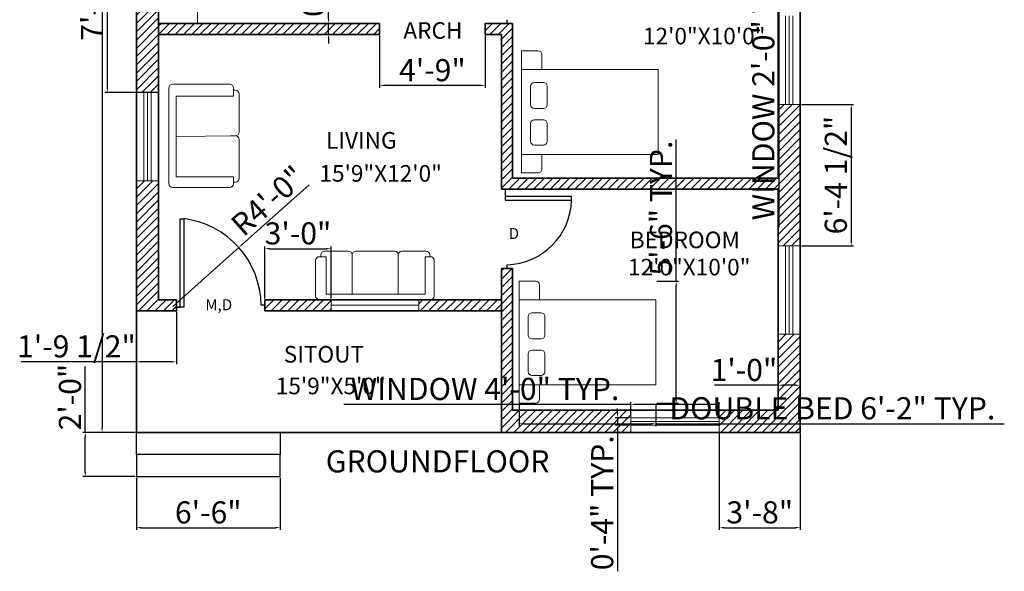
# Model space of a CAD drawing. Units: inches. Extents: x 2105 to 2639, y 1718 to 2373.
# Tile 1 of 2: x 2105 to 2639, y 1718 to 2017. Entities that reach past the tile are written whole.
import ezdxf

# ---------------------------------------------------------------- set-up
doc = ezdxf.new("R2010")
doc.units = ezdxf.units.IN
for name, color, linetype, lineweight in [('A-ANNO-DIMS', 2, 'Continuous', 18), ('A-ANNO-TEXT', 7, 'Continuous', 18), ('A-AREA-IDEN', 7, 'Continuous', 18), ('A-DOOR', 3, 'Continuous', 25), ('A-FLOR-CASE', 9, 'Continuous', 18), ('A-FLOR-STRS', 7, 'Continuous', 25), ('A-FURN', 8, 'Continuous', 18), ('A-GLAZ', 4, 'Continuous', 18), ('A-WALL', 120, 'Continuous', 35), ('A-WALL-PATT', 120, 'Continuous', 13)]:
    doc.layers.add(name, color=color, linetype=linetype, lineweight=lineweight)
doc.styles.get("Standard").update_dxf_attribs({"font": 'arial.ttf'})
doc.dimstyles.new('ISO-25', dxfattribs={"dimtxt": 12, "dimasz": 2.5, "dimexe": 1.25, "dimexo": 0.625, "dimtad": 1, "dimdec": 0, "dimlunit": 3, "dimtxsty": 'Standard', "dimcen": 2.5, "dimadec": 0, "dimazin": 0, "dimtfac": 1, "dimtdec": 0, "dimtmove": 0, "dimatfit": 3, "dimfxl": 1, "dimarcsym": 0})

# ---------------------------------------------------------------- blocks, each defined once
blk = doc.blocks.new('*D2')
at = {"layer": 'A-ANNO-DIMS', "color": 0, "lineweight": -2, "transparency": 16777216}
for p, q in [((2167.25, 2273.29), (2148.02, 2273.29)), ((2149.27, 2270.79), (2149.27, 1795.79)), ((2167.25, 1793.29), (2148.02, 1793.29))]:
    blk.add_line(p, q, dxfattribs=at)
at = {"layer": 'A-ANNO-DIMS', "color": 0, "transparency": 16777216}
for points in [[(2148.85, 2270.79), (2149.68, 2270.79), (2149.27, 2273.29)], [(2148.85, 1795.79), (2149.68, 1795.79), (2149.27, 1793.29)]]:
    blk.add_solid(points, dxfattribs=at)
at = {"layer": 'Defpoints', "color": 0, "transparency": 16777216}
for p in [(2167.87, 2273.29), (2149.27, 1793.29), (2167.87, 1793.29)]:
    blk.add_point(p, dxfattribs=at)
at = {"layer": 'A-ANNO-DIMS', "color": 0, "transparency": 16777216, "insert": (2142.52, 2033.29), "char_height": 12, "attachment_point": 5, "rotation": 90}
blk.add_mtext("40'", dxfattribs=at)
blk = doc.blocks.new('WIN-GLAZ-48IN')
for p, q in [((0, 4), (48, 4)), ((0, 2), (48, 2)), ((0, 0), (48, 0))]:
    blk.add_line(p, q)
blk = doc.blocks.new('DOOR-LEAF-36IN')
for p, q in [((2, 36), (0, 36)), ((0, 36), (0, 0)), ((2, 0), (2, 36)), ((0, 0), (2, 0))]:
    blk.add_line(p, q)
blk = doc.blocks.new('BED-DOUBLE')
for points in [[(0, 56.21), (11, 56.21), (11, 64.21, 0.414214), (9, 66.21), (0, 66.21)], [(6.91, 49.06), (11.92, 49.06, -0.414214), (13.92, 47.06), (13.92, 36.95, -0.414214), (11.92, 34.95), (6.91, 34.95, -0.414214), (4.91, 36.95), (4.91, 47.06, -0.414214)], [(6.91, 28.81), (11.92, 28.81, -0.414214), (13.92, 26.81), (13.92, 17.11, -0.414214), (11.92, 15.11), (6.91, 15.11, -0.414214), (4.91, 17.11), (4.91, 26.81, -0.414214)], [(0, 10), (11, 10), (11, 2, -0.414214), (9, 0), (0, 0)]]:
    blk.add_lwpolyline(points, format="xyb", close=True)
blk.add_lwpolyline([(0, 56.21), (74.08, 56.21), (74.08, 10), (0, 10)], close=True)
blk = doc.blocks.new('*D8')
at = {"layer": 'A-ANNO-DIMS', "color": 0, "lineweight": -2, "transparency": 16777216}
for p, q in [((2435.99, 1808.49), (2280.39, 1808.49)), ((2435.99, 1801.92), (2435.99, 1809.74)), ((2481.49, 1808.49), (2438.49, 1808.49)), ((2483.99, 1801.92), (2483.99, 1809.74))]:
    blk.add_line(p, q, dxfattribs=at)
at = {"layer": 'A-ANNO-DIMS', "color": 0, "transparency": 16777216}
for points in [[(2438.49, 1808.91), (2438.49, 1808.08), (2435.99, 1808.49)], [(2481.49, 1808.91), (2481.49, 1808.08), (2483.99, 1808.49)]]:
    blk.add_solid(points, dxfattribs=at)
at = {"layer": 'Defpoints', "color": 0, "transparency": 16777216}
for p in [(2435.99, 1808.49), (2435.99, 1801.29), (2483.99, 1801.29)]:
    blk.add_point(p, dxfattribs=at)
at = {"layer": 'A-ANNO-DIMS', "color": 0, "transparency": 16777216, "insert": (2356.94, 1815.33), "char_height": 12, "attachment_point": 5}
blk.add_mtext('WINDOW 4\'-0" TYP.', dxfattribs=at)
blk = doc.blocks.new('*D9')
at = {"layer": 'A-ANNO-DIMS', "color": 0, "lineweight": -2, "transparency": 16777216}
for p, q in [((2428.79, 1803.79), (2428.79, 1806.29)), ((2435.37, 1801.29), (2427.54, 1801.29)), ((2428.79, 1801.29), (2428.79, 1797.29)), ((2435.37, 1797.29), (2427.54, 1797.29)), ((2428.79, 1794.79), (2428.79, 1717.9))]:
    blk.add_line(p, q, dxfattribs=at)
at = {"layer": 'A-ANNO-DIMS', "color": 0, "transparency": 16777216}
for points in [[(2428.37, 1803.79), (2429.21, 1803.79), (2428.79, 1801.29)], [(2428.37, 1794.79), (2429.21, 1794.79), (2428.79, 1797.29)]]:
    blk.add_solid(points, dxfattribs=at)
at = {"layer": 'Defpoints', "color": 0, "transparency": 16777216}
for p in [(2435.99, 1801.29), (2428.79, 1797.29), (2435.99, 1797.29)]:
    blk.add_point(p, dxfattribs=at)
at = {"layer": 'A-ANNO-DIMS', "color": 0, "transparency": 16777216, "insert": (2422.04, 1755.09), "char_height": 12, "attachment_point": 5, "rotation": 90}
blk.add_mtext('0\'-4" TYP.', dxfattribs=at)
blk = doc.blocks.new('*D10')
at = {"layer": 'A-ANNO-DIMS', "color": 0, "lineweight": -2, "transparency": 16777216}
for p, q in [((2519.25, 2084.29), (2515.02, 2084.29)), ((2516.27, 2081.79), (2516.27, 2062.79)), ((2519.25, 2060.29), (2515.02, 2060.29)), ((2516.27, 2060.29), (2516.27, 1904.69))]:
    blk.add_line(p, q, dxfattribs=at)
at = {"layer": 'A-ANNO-DIMS', "color": 0, "transparency": 16777216}
for points in [[(2515.86, 2081.79), (2516.69, 2081.79), (2516.27, 2084.29)], [(2515.86, 2062.79), (2516.69, 2062.79), (2516.27, 2060.29)]]:
    blk.add_solid(points, dxfattribs=at)
at = {"layer": 'Defpoints', "color": 0, "transparency": 16777216}
for p in [(2519.87, 2084.29), (2516.27, 2060.29), (2519.87, 2060.29)]:
    blk.add_point(p, dxfattribs=at)
at = {"layer": 'A-ANNO-DIMS', "color": 0, "transparency": 16777216, "insert": (2509.44, 1981.24), "char_height": 12, "attachment_point": 5, "rotation": 90}
blk.add_mtext('WINDOW 2\'-0" TYP.', dxfattribs=at)
blk = doc.blocks.new('*D16')
at = {"layer": 'A-ANNO-DIMS', "color": 0, "lineweight": -2, "transparency": 16777216}
for p, q in [((2375.44, 1808.49), (2375.44, 1796.76)), ((2449.53, 1808.49), (2449.53, 1796.76)), ((2377.94, 1798.01), (2447.03, 1798.01)), ((2449.53, 1798.01), (2638.55, 1798.01))]:
    blk.add_line(p, q, dxfattribs=at)
at = {"layer": 'A-ANNO-DIMS', "color": 0, "transparency": 16777216}
for points in [[(2377.94, 1798.42), (2377.94, 1797.59), (2375.44, 1798.01)], [(2447.03, 1798.42), (2447.03, 1797.59), (2449.53, 1798.01)]]:
    blk.add_solid(points, dxfattribs=at)
at = {"layer": 'Defpoints', "color": 0, "transparency": 16777216}
for p in [(2375.44, 1809.12), (2449.53, 1809.12), (2449.53, 1798.01)]:
    blk.add_point(p, dxfattribs=at)
at = {"layer": 'A-ANNO-DIMS', "color": 0, "transparency": 16777216, "insert": (2545.29, 1804.84), "char_height": 12, "attachment_point": 5}
blk.add_mtext('DOUBLE BED 6\'-2" TYP.', dxfattribs=at)
blk = doc.blocks.new('*D17')
at = {"layer": 'A-ANNO-DIMS', "color": 0, "lineweight": -2, "transparency": 16777216}
for p, q in [((2460.64, 1875.33), (2460.64, 1952.23)), ((2450.15, 1875.33), (2461.89, 1875.33)), ((2460.64, 1811.62), (2460.64, 1872.83)), ((2450.15, 1809.12), (2461.89, 1809.12))]:
    blk.add_line(p, q, dxfattribs=at)
at = {"layer": 'A-ANNO-DIMS', "color": 0, "transparency": 16777216}
for points in [[(2460.22, 1872.83), (2461.06, 1872.83), (2460.64, 1875.33)], [(2460.22, 1811.62), (2461.06, 1811.62), (2460.64, 1809.12)]]:
    blk.add_solid(points, dxfattribs=at)
at = {"layer": 'Defpoints', "color": 0, "transparency": 16777216}
for p in [(2449.53, 1875.33), (2460.64, 1875.33), (2449.53, 1809.12)]:
    blk.add_point(p, dxfattribs=at)
at = {"layer": 'A-ANNO-DIMS', "color": 0, "transparency": 16777216, "insert": (2453.89, 1915.03), "char_height": 12, "attachment_point": 5, "rotation": 90}
blk.add_mtext('5\'-6" TYP.', dxfattribs=at)
blk = doc.blocks.new('*D18')
at = {"layer": 'A-ANNO-DIMS', "color": 0, "lineweight": -2, "transparency": 16777216}
for p, q in [((2167.87, 1768.67), (2167.87, 1740.34)), ((2245.87, 1768.67), (2245.87, 1740.34)), ((2170.37, 1741.59), (2243.37, 1741.59))]:
    blk.add_line(p, q, dxfattribs=at)
at = {"layer": 'A-ANNO-DIMS', "color": 0, "transparency": 16777216}
for points in [[(2170.37, 1742.01), (2170.37, 1741.18), (2167.87, 1741.59)], [(2243.37, 1742.01), (2243.37, 1741.18), (2245.87, 1741.59)]]:
    blk.add_solid(points, dxfattribs=at)
at = {"layer": 'Defpoints', "color": 0, "transparency": 16777216}
for p in [(2167.87, 1769.29), (2245.87, 1769.29), (2245.87, 1741.59)]:
    blk.add_point(p, dxfattribs=at)
at = {"layer": 'A-ANNO-DIMS', "color": 0, "transparency": 16777216, "insert": (2206.87, 1748.34), "char_height": 12, "attachment_point": 5}
blk.add_mtext('6\'-6"', dxfattribs=at)
blk = doc.blocks.new('*D19')
at = {"layer": 'A-ANNO-DIMS', "color": 0, "lineweight": -2, "transparency": 16777216}
for p, q in [((2140.17, 1793.29), (2140.17, 1829.15)), ((2167.25, 1793.29), (2138.92, 1793.29)), ((2140.17, 1771.79), (2140.17, 1790.79)), ((2167.25, 1769.29), (2138.92, 1769.29))]:
    blk.add_line(p, q, dxfattribs=at)
at = {"layer": 'A-ANNO-DIMS', "color": 0, "transparency": 16777216}
for points in [[(2139.76, 1790.79), (2140.59, 1790.79), (2140.17, 1793.29)], [(2139.76, 1771.79), (2140.59, 1771.79), (2140.17, 1769.29)]]:
    blk.add_solid(points, dxfattribs=at)
at = {"layer": 'Defpoints', "color": 0, "transparency": 16777216}
for p in [(2140.17, 1793.29), (2167.87, 1793.29), (2167.87, 1769.29)]:
    blk.add_point(p, dxfattribs=at)
at = {"layer": 'A-ANNO-DIMS', "color": 0, "transparency": 16777216, "insert": (2133.42, 1812.47), "char_height": 12, "attachment_point": 5, "rotation": 90}
blk.add_mtext('2\'-0"', dxfattribs=at)
blk = doc.blocks.new('*D26')
at = {"layer": 'A-ANNO-DIMS', "color": 0, "lineweight": -2, "transparency": 16777216}
for p, q in [((2528.5, 1971.31), (2556.82, 1971.31)), ((2555.57, 1968.81), (2555.57, 1897.09)), ((2528.5, 1894.59), (2556.82, 1894.59))]:
    blk.add_line(p, q, dxfattribs=at)
at = {"layer": 'A-ANNO-DIMS', "color": 0, "transparency": 16777216}
for points in [[(2555.16, 1968.81), (2555.99, 1968.81), (2555.57, 1971.31)], [(2555.16, 1897.09), (2555.99, 1897.09), (2555.57, 1894.59)]]:
    blk.add_solid(points, dxfattribs=at)
at = {"layer": 'Defpoints', "color": 0, "transparency": 16777216}
for p in [(2527.87, 1971.31), (2527.87, 1894.59), (2555.57, 1894.59)]:
    blk.add_point(p, dxfattribs=at)
at = {"layer": 'A-ANNO-DIMS', "color": 0, "transparency": 16777216, "insert": (2548.74, 1932.95), "char_height": 12, "attachment_point": 5, "rotation": 90}
blk.add_mtext('6\'-4 1/2"', dxfattribs=at)
blk = doc.blocks.new('*D27')
at = {"layer": 'A-ANNO-DIMS', "color": 0, "lineweight": -2, "transparency": 16777216}
for p, q in [((2483.99, 1792.67), (2483.99, 1740.34)), ((2527.87, 1792.67), (2527.87, 1740.34)), ((2486.49, 1741.59), (2525.37, 1741.59))]:
    blk.add_line(p, q, dxfattribs=at)
at = {"layer": 'A-ANNO-DIMS', "color": 0, "transparency": 16777216}
for points in [[(2486.49, 1742.01), (2486.49, 1741.18), (2483.99, 1741.59)], [(2525.37, 1742.01), (2525.37, 1741.18), (2527.87, 1741.59)]]:
    blk.add_solid(points, dxfattribs=at)
at = {"layer": 'Defpoints', "color": 0, "transparency": 16777216}
for p in [(2483.99, 1793.29), (2527.87, 1793.29), (2527.87, 1741.59)]:
    blk.add_point(p, dxfattribs=at)
at = {"layer": 'A-ANNO-DIMS', "color": 0, "transparency": 16777216, "insert": (2505.93, 1748.35), "char_height": 12, "attachment_point": 5}
blk.add_mtext('3\'-8"', dxfattribs=at)
blk = doc.blocks.new('*D31')
at = {"layer": 'A-ANNO-DIMS', "color": 0, "lineweight": -2, "transparency": 16777216}
for p, q in [((2179.25, 2070.06), (2150.92, 2070.06)), ((2152.17, 1980.35), (2152.17, 2067.56)), ((2179.25, 1977.85), (2150.92, 1977.85))]:
    blk.add_line(p, q, dxfattribs=at)
at = {"layer": 'A-ANNO-DIMS', "color": 0, "transparency": 16777216}
for points in [[(2151.76, 2067.56), (2152.59, 2067.56), (2152.17, 2070.06)], [(2151.76, 1980.35), (2152.59, 1980.35), (2152.17, 1977.85)]]:
    blk.add_solid(points, dxfattribs=at)
at = {"layer": 'Defpoints', "color": 0, "transparency": 16777216}
for p in [(2152.17, 2070.06), (2179.87, 2070.06), (2179.87, 1977.85)]:
    blk.add_point(p, dxfattribs=at)
at = {"layer": 'A-ANNO-DIMS', "color": 0, "transparency": 16777216, "insert": (2145.42, 2023.95), "char_height": 12, "attachment_point": 5, "rotation": 90}
blk.add_mtext('7\'-8"', dxfattribs=at)
blk = doc.blocks.new('*D32')
at = {"layer": 'A-ANNO-DIMS', "color": 0, "lineweight": -2, "transparency": 16777216}
for p, q in [((2167.87, 1858.67), (2167.87, 1830.34)), ((2189.6, 1858.67), (2189.6, 1830.34)), ((2167.87, 1831.59), (2105.39, 1831.59)), ((2187.1, 1831.59), (2170.37, 1831.59))]:
    blk.add_line(p, q, dxfattribs=at)
at = {"layer": 'A-ANNO-DIMS', "color": 0, "transparency": 16777216}
for points in [[(2170.37, 1832.01), (2170.37, 1831.18), (2167.87, 1831.59)], [(2187.1, 1832.01), (2187.1, 1831.18), (2189.6, 1831.59)]]:
    blk.add_solid(points, dxfattribs=at)
at = {"layer": 'Defpoints', "color": 0, "transparency": 16777216}
for p in [(2167.87, 1859.29), (2189.6, 1859.29), (2167.87, 1831.59)]:
    blk.add_point(p, dxfattribs=at)
at = {"layer": 'A-ANNO-DIMS', "color": 0, "transparency": 16777216, "insert": (2135.38, 1838.42), "char_height": 12, "attachment_point": 5}
blk.add_mtext('1\'-9 1/2"', dxfattribs=at)
blk = doc.blocks.new('*D33')
at = {"layer": 'A-ANNO-DIMS', "color": 0, "lineweight": -2, "transparency": 16777216}
for p, q in [((2237.6, 1865.92), (2237.6, 1894.24)), ((2240.1, 1892.99), (2270.94, 1892.99)), ((2273.44, 1865.92), (2273.44, 1894.24))]:
    blk.add_line(p, q, dxfattribs=at)
at = {"layer": 'A-ANNO-DIMS', "color": 0, "transparency": 16777216}
for points in [[(2240.1, 1893.41), (2240.1, 1892.58), (2237.6, 1892.99)], [(2270.94, 1893.41), (2270.94, 1892.58), (2273.44, 1892.99)]]:
    blk.add_solid(points, dxfattribs=at)
at = {"layer": 'Defpoints', "color": 0, "transparency": 16777216}
for p in [(2273.44, 1892.99), (2237.6, 1865.29), (2273.44, 1865.29)]:
    blk.add_point(p, dxfattribs=at)
at = {"layer": 'A-ANNO-DIMS', "color": 0, "transparency": 16777216, "insert": (2255.52, 1899.75), "char_height": 12, "attachment_point": 5}
blk.add_mtext('3\'-0"', dxfattribs=at)
blk = doc.blocks.new('*D34')
at = {"layer": 'A-ANNO-DIMS', "color": 0, "lineweight": -2, "transparency": 16777216}
for p, q in [((2299.8, 2008.67), (2299.8, 1980.34)), ((2357.02, 2008.67), (2357.02, 1980.34)), ((2354.52, 1981.59), (2302.3, 1981.59))]:
    blk.add_line(p, q, dxfattribs=at)
at = {"layer": 'A-ANNO-DIMS', "color": 0, "transparency": 16777216}
for points in [[(2302.3, 1982.01), (2302.3, 1981.18), (2299.8, 1981.59)], [(2354.52, 1982.01), (2354.52, 1981.18), (2357.02, 1981.59)]]:
    blk.add_solid(points, dxfattribs=at)
at = {"layer": 'Defpoints', "color": 0, "transparency": 16777216}
for p in [(2299.8, 2009.29), (2357.02, 2009.29), (2299.8, 1981.59)]:
    blk.add_point(p, dxfattribs=at)
at = {"layer": 'A-ANNO-DIMS', "color": 0, "transparency": 16777216, "insert": (2328.41, 1988.34), "char_height": 12, "attachment_point": 5}
blk.add_mtext('4\'-9"', dxfattribs=at)
blk = doc.blocks.new('*D37')
at = {"layer": 'A-ANNO-DIMS', "color": 0, "lineweight": -2, "transparency": 16777216}
for p, q in [((2515.87, 1845.96), (2515.87, 1817.64)), ((2527.87, 1845.96), (2527.87, 1817.64)), ((2515.87, 1818.89), (2481.35, 1818.89)), ((2525.37, 1818.89), (2518.37, 1818.89))]:
    blk.add_line(p, q, dxfattribs=at)
at = {"layer": 'A-ANNO-DIMS', "color": 0, "transparency": 16777216}
for points in [[(2518.37, 1819.3), (2518.37, 1818.47), (2515.87, 1818.89)], [(2525.37, 1819.3), (2525.37, 1818.47), (2527.87, 1818.89)]]:
    blk.add_solid(points, dxfattribs=at)
at = {"layer": 'Defpoints', "color": 0, "transparency": 16777216}
for p in [(2515.87, 1846.59), (2527.87, 1846.59), (2515.87, 1818.89)]:
    blk.add_point(p, dxfattribs=at)
at = {"layer": 'A-ANNO-DIMS', "color": 0, "transparency": 16777216, "insert": (2497.36, 1825.64), "char_height": 12, "attachment_point": 5}
blk.add_mtext('1\'-0"', dxfattribs=at)
blk = doc.blocks.new('*D38')
at = {"layer": 'A-ANNO-DIMS', "color": 0, "lineweight": -2, "transparency": 16777216}
for p, q in [((2272.1, 2017.79), (2272.1, 2053.44)), ((2299.18, 2015.29), (2270.85, 2015.29)), ((2272.1, 2009.29), (2272.1, 2015.29)), ((2299.18, 2009.29), (2270.85, 2009.29)), ((2272.1, 2006.79), (2272.1, 2004.29))]:
    blk.add_line(p, q, dxfattribs=at)
at = {"layer": 'A-ANNO-DIMS', "color": 0, "transparency": 16777216}
for points in [[(2271.69, 2017.79), (2272.52, 2017.79), (2272.1, 2015.29)], [(2271.69, 2006.79), (2272.52, 2006.79), (2272.1, 2009.29)]]:
    blk.add_solid(points, dxfattribs=at)
at = {"layer": 'Defpoints', "color": 0, "transparency": 16777216}
for p in [(2272.1, 2015.29), (2299.8, 2015.29), (2299.8, 2009.29)]:
    blk.add_point(p, dxfattribs=at)
at = {"layer": 'A-ANNO-DIMS', "color": 0, "transparency": 16777216, "insert": (2265.35, 2036.87), "char_height": 12, "attachment_point": 5, "rotation": 90}
blk.add_mtext('0\'-6"', dxfattribs=at)
blk = doc.blocks.new('*D41')
at = {"layer": 'A-ANNO-DIMS', "color": 0, "lineweight": -2, "transparency": 16777216}
for p, q in [((2261.51, 1927.71), (2225.26, 1895.32)), ((2187.61, 1861.67), (2223.4, 1893.65))]:
    blk.add_line(p, q, dxfattribs=at)
at = {"layer": 'A-ANNO-DIMS', "color": 0, "transparency": 16777216}
blk.add_solid([(2224.99, 1895.63), (2225.54, 1895.01), (2223.4, 1893.65)], dxfattribs=at)
at = {"layer": 'Defpoints', "color": 0, "transparency": 16777216}
for p in [(2223.4, 1893.65), (2187.61, 1861.67)]:
    blk.add_point(p, dxfattribs=at)
at = {"layer": 'A-ANNO-DIMS', "color": 0, "transparency": 16777216, "insert": (2240.37, 1917.88), "char_height": 12, "attachment_point": 5, "rotation": 41.7849}
blk.add_mtext('R4\'-0"', dxfattribs=at)

msp = doc.modelspace()

# ---------------------------------------------------------------- hatches: boundary and pattern name
at = {"layer": 'A-WALL-PATT'}
h = msp.add_hatch(dxfattribs=at)
h.set_pattern_fill('ANSI31', color=256)
h.paths.add_polyline_path([(2179.87, 2070.06), (2167.87, 2070.06), (2167.87, 1977.85), (2179.87, 1977.85)])
h = msp.add_hatch(dxfattribs=at)
h.set_pattern_fill('ANSI31', color=256)
h.paths.add_polyline_path([(2299.8, 2015.29), (2179.87, 2015.29), (2179.87, 2009.29), (2299.8, 2009.29)])
h = msp.add_hatch(dxfattribs=at)
h.set_pattern_fill('ANSI31', color=256)
h.paths.add_polyline_path([(2371.87, 2015.29), (2357.02, 2015.29), (2357.02, 2009.29), (2365.87, 2009.29), (2365.87, 1925.29), (2367.87, 1925.29), (2371.87, 1925.29), (2515.87, 1925.29), (2515.87, 1894.59), (2527.87, 1894.59), (2527.87, 1971.31), (2515.87, 1971.31), (2515.87, 1931.29), (2371.87, 1931.29)])
h = msp.add_hatch(dxfattribs=at)
h.set_pattern_fill('ANSI31', color=256)
h.paths.add_polyline_path([(2189.6, 1861.29), (2189.6, 1865.29), (2179.87, 1865.29), (2179.87, 1929.85), (2167.87, 1929.85), (2167.87, 1859.29), (2179.87, 1859.29), (2189.6, 1859.29)])
h = msp.add_hatch(dxfattribs=at)
h.set_pattern_fill('ANSI31', color=256)
h.paths.add_polyline_path([(2435.99, 1805.29), (2371.87, 1805.29), (2371.87, 1882.29), (2365.87, 1882.29), (2365.87, 1805.29), (2365.87, 1793.29), (2435.99, 1793.29)])
h = msp.add_hatch(dxfattribs=at)
h.set_pattern_fill('ANSI31', color=256)
h.paths.add_polyline_path([(2273.44, 1865.29), (2237.6, 1865.29), (2237.6, 1859.29), (2273.44, 1859.29)])
h = msp.add_hatch(dxfattribs=at)
h.set_pattern_fill('ANSI31', color=256)
h.paths.add_polyline_path([(2365.87, 1865.29), (2321.01, 1865.29), (2321.01, 1859.29), (2365.87, 1859.29)])
h = msp.add_hatch(dxfattribs=at)
h.set_pattern_fill('ANSI31', color=256)
h.paths.add_polyline_path([(2527.87, 1846.59), (2515.87, 1846.59), (2515.87, 1805.29), (2483.99, 1805.29), (2483.99, 1793.29), (2527.87, 1793.29)])

# ---------------------------------------------------------------- linework, layer by layer
at = {"layer": 'A-DOOR'}
for p, q in [((2368.87, 2015.29), (2368.87, 2017.29)), ((2371.87, 2015.29), (2368.87, 2015.29)), ((2365.87, 1925.29), (2367.87, 1925.29)), ((2367.87, 1925.29), (2367.87, 1921.29)), ((2191.6, 1861.29), (2191.6, 1909.29)), ((2191.6, 1909.29), (2193.6, 1909.29)), ((2193.6, 1909.29), (2193.6, 1861.29)), ((2368.87, 1882.29), (2368.87, 1884.29)), ((2189.6, 1859.29), (2189.6, 1861.29)), ((2189.6, 1861.29), (2191.6, 1861.29)), ((2193.6, 1861.29), (2190.6, 1861.29)), ((2237.6, 1862.29), (2235.6, 1862.29))]:
    msp.add_line(p, q, dxfattribs=at)
for centre, radius, start, end in [((2367.89, 1920.28), 36, 271.5702, 358.4298), ((2187.61, 1861.67), 48, 0.7449, 82.8241)]:
    msp.add_arc(centre, radius, start, end, dxfattribs=at)
at = {"layer": 'A-FLOR-CASE'}
msp.add_lwpolyline([(2179.87, 2015.29), (2201.1, 2015.29), (2201.1, 2060.06), (2179.87, 2060.06)], close=True, dxfattribs=at)
at = {"layer": 'A-FLOR-STRS'}
for p, q in [((2167.87, 1793.29), (2245.87, 1793.29)), ((2167.87, 1781.29), (2167.87, 1793.29)), ((2245.87, 1793.29), (2245.87, 1781.29)), ((2245.87, 1781.29), (2167.87, 1781.29)), ((2167.87, 1781.29), (2167.87, 1769.29)), ((2245.87, 1769.29), (2245.87, 1781.29)), ((2245.87, 1781.29), (2245.87, 1781.29)), ((2167.87, 1769.29), (2245.87, 1769.29))]:
    msp.add_line(p, q, dxfattribs=at)
at = {"layer": 'A-FURN'}
for p, q in [((2220.58, 1979.04), (2221.58, 1979.04)), ((2223.58, 1977.04), (2223.58, 1956.27)), ((2221.55, 1954.27), (2189.55, 1953.83)), ((2221.6, 1954.27), (2218.87, 1954.23)), ((2223.58, 1931.09), (2223.58, 1952.27)), ((2220.58, 1929.09), (2221.58, 1929.09)), ((2324.94, 1891.66), (2311.94, 1891.66)), ((2267.91, 1888.66), (2267.91, 1889.66)), ((2309.94, 1889.66), (2309.94, 1868.36)), ((2326.94, 1888.66), (2326.94, 1889.66))]:
    msp.add_line(p, q, dxfattribs=at)
for points in [[(2220.58, 1931.91), (2220.58, 1928.27, -0.414214), (2218.58, 1926.27), (2187.47, 1926.27, -0.414214), (2185.47, 1928.27), (2185.47, 1980.33, -0.414214), (2187.47, 1982.33), (2218.58, 1982.33, -0.414214), (2220.58, 1980.33), (2220.58, 1975.75)], [(2284.91, 1868.36), (2284.91, 1889.66, -0.414214), (2286.91, 1891.66), (2307.94, 1891.66, -0.414214), (2309.94, 1889.66), (2309.94, 1868.36), (2284.91, 1868.36), (2284.91, 1889.66, 0.414214), (2282.91, 1891.66), (2269.91, 1891.66)], [(2324.51, 1888.66), (2327.36, 1888.66, -0.414214), (2329.36, 1886.66), (2329.36, 1867.29, -0.414214), (2327.36, 1865.29), (2267.09, 1865.29, -0.414214), (2265.09, 1867.29), (2265.09, 1886.66, -0.414214), (2267.09, 1888.66), (2270.74, 1888.66)]]:
    msp.add_lwpolyline(points, format="xyb", dxfattribs=at)
for points in [[(2220.58, 1975.75), (2189.55, 1975.75), (2189.55, 1931.91), (2220.58, 1931.91)], [(2324.51, 1888.66), (2324.51, 1868.36), (2270.74, 1868.36), (2270.74, 1888.66)]]:
    msp.add_lwpolyline(points, dxfattribs=at)
for centre, start, end in [((2221.58, 1977.04), 0, 90), ((2221.58, 1952.27), 360, 90.7909), ((2221.58, 1956.27), 270.7909, 0), ((2221.58, 1931.09), 270, 360), ((2269.91, 1889.66), 90, 180), ((2311.94, 1889.66), 90, 180), ((2324.94, 1889.66), 0, 90)]:
    msp.add_arc(centre, 2, start, end, dxfattribs=at)
at = {"layer": 'A-GLAZ'}
for p, q in [((2167.87, 1977.85), (2179.87, 1977.85)), ((2527.87, 1971.31), (2515.87, 1971.31)), ((2167.87, 1929.85), (2179.87, 1929.85)), ((2527.87, 1894.59), (2515.87, 1894.59)), ((2273.44, 1865.29), (2273.44, 1859.29)), ((2321.01, 1865.29), (2321.01, 1859.29)), ((2273.44, 1862.29), (2321.01, 1862.29)), ((2527.87, 1846.59), (2515.87, 1846.59)), ((2435.99, 1793.29), (2435.99, 1805.29)), ((2483.99, 1793.29), (2483.99, 1805.29))]:
    msp.add_line(p, q, dxfattribs=at)
at = {"layer": 'A-WALL'}
for p, q in [((2179.87, 1865.29), (2179.87, 2129.29)), ((2515.87, 2054.29), (2515.87, 1931.29)), ((2179.87, 2015.29), (2299.8, 2015.29)), ((2299.8, 2015.29), (2299.8, 2009.29)), ((2357.02, 2015.29), (2371.87, 2015.29)), ((2357.02, 2015.29), (2357.02, 2009.29)), ((2371.87, 1931.29), (2371.87, 2015.29)), ((2179.87, 2009.29), (2299.8, 2009.29)), ((2357.02, 2009.29), (2365.87, 2009.29)), ((2365.87, 1925.29), (2365.87, 2009.29)), ((2515.87, 1931.29), (2371.87, 1931.29)), ((2371.87, 1925.29), (2365.87, 1925.29)), ((2515.87, 1925.29), (2371.87, 1925.29)), ((2515.87, 1925.29), (2515.87, 1805.29)), ((2365.87, 1805.29), (2365.87, 1882.29)), ((2371.87, 1882.29), (2365.87, 1882.29)), ((2371.87, 1805.29), (2371.87, 1882.29)), ((2179.87, 1865.29), (2189.6, 1865.29)), ((2189.6, 1865.29), (2189.6, 1859.29)), ((2237.6, 1865.29), (2237.6, 1859.29)), ((2237.6, 1865.29), (2365.87, 1865.29)), ((2179.87, 1859.29), (2167.87, 1859.29)), ((2179.87, 1859.29), (2189.6, 1859.29)), ((2237.6, 1859.29), (2365.87, 1859.29)), ((2365.87, 1805.29), (2365.87, 1793.29)), ((2515.87, 1805.29), (2371.87, 1805.29))]:
    msp.add_line(p, q, dxfattribs=at)
msp.add_lwpolyline([(2167.87, 2172.29), (2167.87, 2273.29), (2527.87, 2273.29), (2527.87, 1793.29), (2167.87, 1793.29), (2167.87, 2129.29)], dxfattribs=at)

# ---------------------------------------------------------------- block references
at = {"layer": 'A-DOOR', "rotation": 89.99999999999785}
msp.add_blockref('DOOR-LEAF-36IN', (2403.87, 1919.29), dxfattribs=at)
at = {"layer": 'A-FURN', "rotation": 0.0004994955271128}
msp.add_blockref('BED-DOUBLE', (2376.79, 1934.13), dxfattribs=at)
at = {"layer": 'A-FURN'}
msp.add_blockref('BED-DOUBLE', (2375.44, 1809.12), dxfattribs=at)
at = {"layer": 'A-GLAZ'}
for p, rotation in [((2519.87, 2019.31), 270.0000000000023), ((2175.87, 1929.85), 90.00000000000097), ((2519.87, 1894.59), 270.0000000000021), ((2483.99, 1801.29), 180)]:
    msp.add_blockref('WIN-GLAZ-48IN', p, dxfattribs=dict(at, rotation=rotation))

# ---------------------------------------------------------------- texts
at = {"layer": 'A-ANNO-TEXT'}
for tag, p, height in [('ARCH', (2312.67, 2006.92), 9), ('D', (2369.77, 1898.27), 6), ('M,D', (2205.29, 1859.59), 6), ('GROUNDFLOOR', (2270.57, 1771.58), 12)]:
    msp.add_attdef(tag, p, '', height=height, dxfattribs=at)
at = {"layer": 'A-AREA-IDEN'}
for tag, p in [('12\'0"X10\'0"', (2442.61, 2003.9)), ('LIVING', (2270.74, 1947.3)), ('15\'9"X12\'0"', (2267.16, 1929.38)), ('BEDROOM', (2435.44, 1893.27)), ('12\'0"X10\'0"', (2434.49, 1878.5)), ('SITOUT', (2247.79, 1831.2)), ('15\'9"X5\'0"', (2243.49, 1814))]:
    msp.add_attdef(tag, p, '', height=9, dxfattribs=at)

# ---------------------------------------------------------------- dimensions: what is measured, and where the dimension line sits
at = {"layer": 'A-ANNO-DIMS'}
for base, p1, p2, angle, override, picture, middle in [((2149.27, 1793.29), (2167.87, 2273.29), (2167.87, 1793.29), 90, {"dimclrd": 0, "dimclre": 0, "dimclrt": 0}, '*D2', (2142.52, 2033.29)), ((2152.17, 2070.06), (2179.87, 1977.85), (2179.87, 2070.06), 90, {"dimdec": 1, "dimlfac": 1, "dimrnd": 0, "dimzin": 1, "dimdsep": 46, "dimlunit": 4, "dimfrac": 2}, '*D31', (2145.42, 2023.95)), ((2272.1, 2015.29), (2299.8, 2009.29), (2299.8, 2015.29), 90, {"dimdec": 1, "dimlfac": 1, "dimrnd": 0, "dimzin": 1, "dimdsep": 46, "dimlunit": 4, "dimfrac": 2}, '*D38', (2265.35, 2036.87)), ((2299.8, 1981.59), (2357.02, 2009.29), (2299.8, 2009.29), 180, {"dimdec": 1, "dimlfac": 1, "dimrnd": 0, "dimzin": 1, "dimdsep": 46, "dimlunit": 4, "dimfrac": 2}, '*D34', (2328.41, 1988.34)), ((2555.57, 1894.59), (2527.87, 1971.31), (2527.87, 1894.59), 90, {"dimdec": 1, "dimlfac": 1, "dimrnd": 0, "dimzin": 1, "dimdsep": 46, "dimlunit": 4, "dimfrac": 2}, '*D26', (2548.74, 1932.95)), ((2167.87, 1831.59), (2189.6, 1859.29), (2167.87, 1859.29), 180, {"dimdec": 1, "dimlfac": 1, "dimrnd": 0, "dimzin": 1, "dimdsep": 46, "dimlunit": 4, "dimfrac": 2}, '*D32', (2135.38, 1838.42)), ((2515.87, 1818.89), (2527.87, 1846.59), (2515.87, 1846.59), 180, {"dimdec": 1, "dimlfac": 1, "dimrnd": 0, "dimzin": 1, "dimdsep": 46, "dimlunit": 4, "dimfrac": 2}, '*D37', (2497.36, 1825.64)), ((2140.17, 1793.29), (2167.87, 1769.29), (2167.87, 1793.29), 90, {"dimdec": 1, "dimlfac": 1, "dimrnd": 0, "dimzin": 1, "dimdsep": 46, "dimlunit": 4, "dimfrac": 2}, '*D19', (2133.42, 1812.47))]:
    dim = msp.add_linear_dim(base=base, p1=p1, p2=p2, angle=angle, dimstyle='ISO-25', override=override, dxfattribs=at)
    dim.commit()
    dim.dimension.update_dxf_attribs({"geometry": picture, "text_midpoint": middle})
for base, p1, p2, angle, text, picture, middle in [((2516.27, 2060.29), (2519.87, 2084.29), (2519.87, 2060.29), 270, 'WINDOW <> TYP.', '*D10', (2509.44, 1981.24)), ((2460.64, 1875.33), (2449.53, 1809.12), (2449.53, 1875.33), 90, '<> TYP.', '*D17', (2453.89, 1915.03)), ((2435.99, 1808.49), (2483.99, 1801.29), (2435.99, 1801.29), 180, 'WINDOW <> TYP.', '*D8', (2356.94, 1815.33)), ((2428.79, 1797.29), (2435.99, 1801.29), (2435.99, 1797.29), 270, '<> TYP.', '*D9', (2422.04, 1755.09))]:
    dim = msp.add_linear_dim(base=base, p1=p1, p2=p2, angle=angle, text=text, dimstyle='ISO-25', override={"dimdec": 1, "dimlfac": 1, "dimrnd": 0, "dimzin": 1, "dimdsep": 46, "dimlunit": 4, "dimfrac": 2}, dxfattribs=at)
    dim.commit()
    dim.dimension.update_dxf_attribs({"geometry": picture, "text_midpoint": middle})
dim = msp.add_radius_dim(center=(2187.61, 1861.67), mpoint=(2223.4, 1893.65), dimstyle='ISO-25', override={"dimdec": 1, "dimlfac": 1, "dimrnd": 0, "dimzin": 1, "dimdsep": 46, "dimlunit": 4, "dimfrac": 2}, dxfattribs=at)
dim.commit()
dim.dimension.update_dxf_attribs({"geometry": '*D41', "text_midpoint": (2244.87, 1912.84), "dimtype": 164})
for base, p1, p2, picture, middle in [((2273.44, 1892.99), (2237.6, 1865.29), (2273.44, 1865.29), '*D33', (2255.52, 1899.75)), ((2527.87, 1741.59), (2483.99, 1793.29), (2527.87, 1793.29), '*D27', (2505.93, 1748.35)), ((2245.87, 1741.59), (2167.87, 1769.29), (2245.87, 1769.29), '*D18', (2206.87, 1748.34))]:
    dim = msp.add_linear_dim(base=base, p1=p1, p2=p2, dimstyle='ISO-25', override={"dimdec": 1, "dimlfac": 1, "dimrnd": 0, "dimzin": 1, "dimdsep": 46, "dimlunit": 4, "dimfrac": 2}, dxfattribs=at)
    dim.commit()
    dim.dimension.update_dxf_attribs({"geometry": picture, "text_midpoint": middle})
dim = msp.add_linear_dim(base=(2449.53, 1798.01), p1=(2375.44, 1809.12), p2=(2449.53, 1809.12), text='DOUBLE BED <> TYP.', dimstyle='ISO-25', override={"dimdec": 1, "dimlfac": 1, "dimrnd": 0, "dimzin": 1, "dimdsep": 46, "dimlunit": 4, "dimfrac": 2}, dxfattribs=at)
dim.commit()
dim.dimension.update_dxf_attribs({"geometry": '*D16', "text_midpoint": (2545.29, 1804.84)})

doc.saveas('drawing.dxf')
